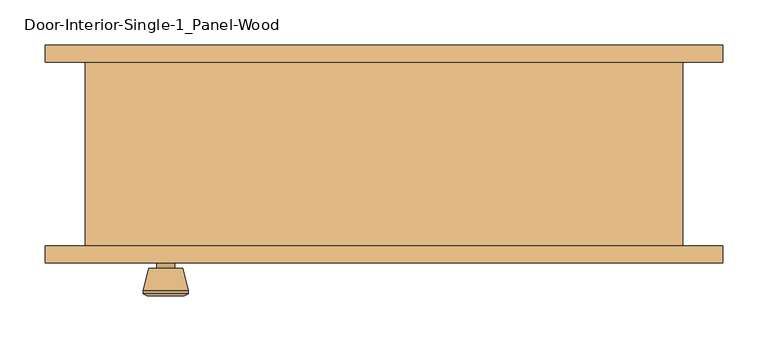
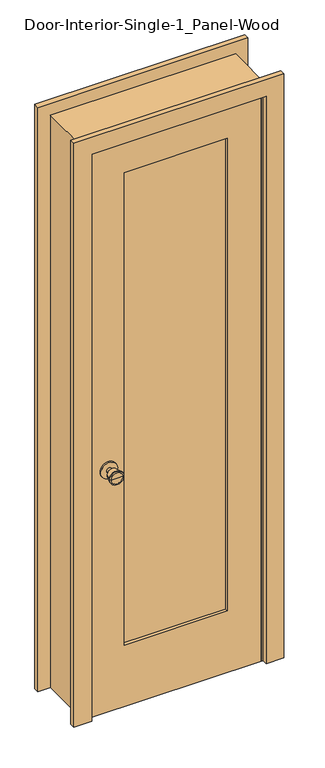
"""IFC4 building model written with IfcOpenShell, lengths in millimetres: door geometry, Door-Interior-Single-1_Panel-Wood."""

from ifc_helpers import new_model, si_unit, point, frame, frame_2d, origin, place, context, project, spatial, polyline, circle_curve, trimmed, segment, composite_curve, outline, extrude, faceted_brep, source, transform, mapped, element, save
from ifc_brep_helpers import plane_surface, cylinder_surface, revolved_surface, advanced_brep


def door_interior_single_1_panel_wood_a1a047a4(model_context):
    return source(origin(), model_context, "Body", "SolidModel", [
        advanced_brep(
        [(-241.3, -57.5, 914.4), (-251.3, -57.5, 914.4), (-231.3, -57.5, 914.4), (-220.8241324, -8.5, 914.4), (-261.7758676, -8.5, 914.4), (-241.3, -8.5, 914.4), (-216.3, -10.3278681, 914.4), (-266.3, -10.3278681, 914.4), (-216.3, -13.7915463, 914.4), (-266.3, -13.7915463, 914.4), (-222.663764, -38.5, 914.4), (-259.936236, -38.5, 914.4), (-231.3, -38.5, 914.4), (-251.3, -38.5, 914.4)],
        [
            (0, 1),
            (1, 2, circle_curve(frame((-241.3, -57.5, 914.4), z_axis=(0.0, -1.0, 0.0), x_axis=(-1.0, 0.0, 0.0)), 10.0)),
            (2, 0),
            (2, 1, circle_curve(frame((-241.3, -57.5, 914.4), z_axis=(0.0, -1.0, 0.0), x_axis=(-1.0, 0.0, 0.0)), 10.0)),
            (3, 4, circle_curve(frame((-241.3, -8.5, 914.4), z_axis=(0.0, 1.0, 0.0), x_axis=(-1.0, 0.0, 0.0)), 20.4758676)),
            (4, 5),
            (5, 3),
            (4, 3, circle_curve(frame((-241.3, -8.5, 914.4), z_axis=(0.0, 1.0, 0.0), x_axis=(-1.0, 0.0, 0.0)), 20.4758676)),
            (6, 7, circle_curve(frame((-241.3, -10.3278681, 914.4), z_axis=(0.0, 1.0, 0.0), x_axis=(-1.0, 0.0, 0.0)), 25.0)),
            (7, 4),
            (3, 6),
            (7, 6, circle_curve(frame((-241.3, -10.3278681, 914.4), z_axis=(0.0, 1.0, 0.0), x_axis=(-1.0, 0.0, 0.0)), 25.0)),
            (8, 9, circle_curve(frame((-241.3, -13.7915463, 914.4), z_axis=(0.0, 1.0, 0.0), x_axis=(-1.0, 0.0, 0.0)), 25.0)),
            (9, 7),
            (6, 8),
            (9, 8, circle_curve(frame((-241.3, -13.7915463, 914.4), z_axis=(0.0, 1.0, 0.0), x_axis=(-1.0, 0.0, 0.0)), 25.0)),
            (10, 11, circle_curve(frame((-241.3, -38.5, 914.4), z_axis=(0.0, 1.0, 0.0), x_axis=(-1.0, 0.0, 0.0)), 18.636236)),
            (11, 9),
            (8, 10),
            (11, 10, circle_curve(frame((-241.3, -38.5, 914.4), z_axis=(0.0, 1.0, 0.0), x_axis=(-1.0, 0.0, 0.0)), 18.636236)),
            (12, 13, circle_curve(frame((-241.3, -38.5, 914.4), z_axis=(0.0, 1.0, 0.0), x_axis=(-1.0, 0.0, 0.0)), 10.0)),
            (13, 11),
            (10, 12),
            (13, 12, circle_curve(frame((-241.3, -38.5, 914.4), z_axis=(0.0, 1.0, 0.0), x_axis=(-1.0, 0.0, 0.0)), 10.0)),
            (1, 13),
            (12, 2),
        ],
        [
            plane_surface(frame((-241.3, -57.5, 914.4), z_axis=(0.0, -1.0, 0.0), x_axis=(-1.0, 0.0, 0.0))),
            plane_surface(frame((-241.3, -8.5, 914.4), z_axis=(0.0, 1.0, 0.0), x_axis=(-1.0, 0.0, 0.0))),
            revolved_surface(polyline([(-261.7758676, -8.5, 914.4), (-266.3, -10.3278681, 914.4)]), (-241.3, -57.5, 914.4), (0.0, -1.0, 0.0)),
            cylinder_surface(frame((-241.3, -57.5, 914.4), z_axis=(0.0, -1.0, 0.0), x_axis=(-1.0, 0.0, 0.0)), 25.0),
            revolved_surface(polyline([(-266.3, -13.7915463, 914.4), (-259.936236, -38.5, 914.4)]), (-241.3, -57.5, 914.4), (0.0, -1.0, 0.0)),
            plane_surface(frame((-241.3, -38.5, 914.4), z_axis=(0.0, -1.0, 0.0), x_axis=(-1.0, 0.0, 0.0))),
            cylinder_surface(frame((-241.3, -57.5, 914.4), z_axis=(0.0, -1.0, 0.0), x_axis=(-1.0, 0.0, 0.0)), 10.0),
        ],
        [
            (0, [[1, 2, 3]]),
            (0, [[-3, 4, -1]]),
            (1, [[5, 6, 7]]),
            (1, [[8, -7, -6]]),
            (2, [[9, 10, -5, 11]]),
            (2, [[12, -11, -8, -10]]),
            (3, [[13, 14, -9, 15]]),
            (3, [[16, -15, -12, -14]]),
            (4, [[17, 18, -13, 19]]),
            (4, [[20, -19, -16, -18]]),
            (5, [[21, 22, -17, 23]]),
            (5, [[24, -23, -20, -22]]),
            (6, [[-2, 25, -21, 26]]),
            (6, [[-4, -26, -24, -25]]),
        ],
    ),
        extrude(outline(composite_curve([segment(trimmed(circle_curve(frame_2d((914.4, -241.3)), 30.0), [point((914.4, -271.3))], [point((914.4, -211.3))], False, "CARTESIAN"), True, "CONTINUOUS"), segment(trimmed(circle_curve(frame_2d((914.4, -241.3)), 30.0), [point((914.4, -211.3))], [point((914.4, -271.3))], False, "CARTESIAN"), True, "CONTINUOUS")], self_intersect=False)), frame((0.0, -63.5, 0.0), z_axis=(0.0, 1.0, 0.0), x_axis=(0.0, 0.0, 1.0)), (0.0, 0.0, 1.0), 6.0),
        advanced_brep(
        [(-241.3, -104.425, 914.4), (-231.3, -104.425, 914.4), (-251.3, -104.425, 914.4), (-220.8241324, -153.425, 914.4), (-241.3, -153.425, 914.4), (-261.7758676, -153.425, 914.4), (-216.3, -151.5971319, 914.4), (-266.3, -151.5971319, 914.4), (-216.3, -148.1334537, 914.4), (-266.3, -148.1334537, 914.4), (-222.663764, -123.425, 914.4), (-259.936236, -123.425, 914.4), (-231.3, -123.425, 914.4), (-251.3, -123.425, 914.4)],
        [
            (0, 1),
            (1, 2, circle_curve(frame((-241.3, -104.425, 914.4), z_axis=(0.0, 1.0, 0.0), x_axis=(-1.0, 0.0, 0.0)), 10.0)),
            (2, 0),
            (2, 1, circle_curve(frame((-241.3, -104.425, 914.4), z_axis=(0.0, 1.0, 0.0), x_axis=(-1.0, 0.0, 0.0)), 10.0)),
            (3, 4),
            (4, 5),
            (5, 3, circle_curve(frame((-241.3, -153.425, 914.4), z_axis=(0.0, -1.0, 0.0), x_axis=(-1.0, 0.0, 0.0)), 20.4758676)),
            (3, 5, circle_curve(frame((-241.3, -153.425, 914.4), z_axis=(0.0, -1.0, 0.0), x_axis=(-1.0, 0.0, 0.0)), 20.4758676)),
            (6, 3),
            (5, 7),
            (7, 6, circle_curve(frame((-241.3, -151.5971319, 914.4), z_axis=(0.0, -1.0, 0.0), x_axis=(-1.0, 0.0, 0.0)), 25.0)),
            (6, 7, circle_curve(frame((-241.3, -151.5971319, 914.4), z_axis=(0.0, -1.0, 0.0), x_axis=(-1.0, 0.0, 0.0)), 25.0)),
            (8, 6),
            (7, 9),
            (9, 8, circle_curve(frame((-241.3, -148.1334537, 914.4), z_axis=(0.0, -1.0, 0.0), x_axis=(-1.0, 0.0, 0.0)), 25.0)),
            (8, 9, circle_curve(frame((-241.3, -148.1334537, 914.4), z_axis=(0.0, -1.0, 0.0), x_axis=(-1.0, 0.0, 0.0)), 25.0)),
            (10, 8),
            (9, 11),
            (11, 10, circle_curve(frame((-241.3, -123.425, 914.4), z_axis=(0.0, -1.0, 0.0), x_axis=(-1.0, 0.0, 0.0)), 18.636236)),
            (10, 11, circle_curve(frame((-241.3, -123.425, 914.4), z_axis=(0.0, -1.0, 0.0), x_axis=(-1.0, 0.0, 0.0)), 18.636236)),
            (12, 10),
            (11, 13),
            (13, 12, circle_curve(frame((-241.3, -123.425, 914.4), z_axis=(0.0, -1.0, 0.0), x_axis=(-1.0, 0.0, 0.0)), 10.0)),
            (12, 13, circle_curve(frame((-241.3, -123.425, 914.4), z_axis=(0.0, -1.0, 0.0), x_axis=(-1.0, 0.0, 0.0)), 10.0)),
            (1, 12),
            (13, 2),
        ],
        [
            plane_surface(frame((-241.3, -104.425, 914.4), z_axis=(0.0, 1.0, 0.0), x_axis=(-1.0, 0.0, 0.0))),
            plane_surface(frame((-241.3, -153.425, 914.4), z_axis=(0.0, -1.0, 0.0), x_axis=(-1.0, 0.0, 0.0))),
            revolved_surface(polyline([(-261.7758676, -153.425, 914.4), (-266.3, -151.5971319, 914.4)]), (-241.3, -104.425, 914.4), (0.0, 1.0, 0.0)),
            cylinder_surface(frame((-241.3, -104.425, 914.4), z_axis=(0.0, 1.0, 0.0), x_axis=(-1.0, 0.0, 0.0)), 25.0),
            revolved_surface(polyline([(-266.3, -148.1334537, 914.4), (-259.936236, -123.425, 914.4)]), (-241.3, -104.425, 914.4), (0.0, 1.0, 0.0)),
            plane_surface(frame((-241.3, -123.425, 914.4), z_axis=(0.0, 1.0, 0.0), x_axis=(-1.0, 0.0, 0.0))),
            cylinder_surface(frame((-241.3, -104.425, 914.4), z_axis=(0.0, 1.0, 0.0), x_axis=(-1.0, 0.0, 0.0)), 10.0),
        ],
        [
            (0, [[1, 2, 3]]),
            (0, [[-3, 4, -1]]),
            (1, [[5, 6, 7]]),
            (1, [[-6, -5, 8]]),
            (2, [[9, -7, 10, 11]]),
            (2, [[-10, -8, -9, 12]]),
            (3, [[13, -11, 14, 15]]),
            (3, [[-14, -12, -13, 16]]),
            (4, [[17, -15, 18, 19]]),
            (4, [[-18, -16, -17, 20]]),
            (5, [[21, -19, 22, 23]]),
            (5, [[-22, -20, -21, 24]]),
            (6, [[25, -23, 26, -2]]),
            (6, [[-26, -24, -25, -4]]),
        ],
    ),
        extrude(outline(composite_curve([segment(trimmed(circle_curve(frame_2d((914.4, -241.3)), 30.0), [point((914.4, -271.3))], [point((914.4, -211.3))], False, "CARTESIAN"), True, "CONTINUOUS"), segment(trimmed(circle_curve(frame_2d((914.4, -241.3)), 30.0), [point((914.4, -211.3))], [point((914.4, -271.3))], False, "CARTESIAN"), True, "CONTINUOUS")], self_intersect=False)), frame((0.0, -104.425, 0.0), z_axis=(0.0, 1.0, 0.0), x_axis=(0.0, 0.0, 1.0)), (0.0, 0.0, 1.0), 6.0),
        faceted_brep([(330.2, -98.425, 0.0), (304.8, -98.425, 0.0), (304.8, -63.5, 0.0), (292.1, -63.5, 0.0), (292.1, -28.575, 0.0), (304.8, -28.575, 0.0), (304.8, 104.775, 0.0), (330.2, 104.775, 0.0), (330.2, 104.775, 2159.0), (330.2, -98.425, 2159.0), (304.8, 104.775, 2133.6), (-304.8, 104.775, 2133.6), (-304.8, 104.775, 0.0), (-330.2, 104.775, 0.0), (-330.2, 104.775, 2159.0), (304.8, -28.575, 2133.6), (292.1, -28.575, 2120.9), (-292.1, -28.575, 2120.9), (-292.1, -28.575, 0.0), (-304.8, -28.575, 0.0), (-304.8, -28.575, 2133.6), (292.1, -63.5, 2120.9), (304.8, -63.5, 2133.6), (-304.8, -63.5, 2133.6), (-304.8, -63.5, 0.0), (-292.1, -63.5, 0.0), (-292.1, -63.5, 2120.9), (304.8, -98.425, 2133.6), (-330.2, -98.425, 2159.0), (-330.2, -98.425, 0.0), (-304.8, -98.425, 0.0), (-304.8, -98.425, 2133.6)], [[[0, 1, 2, 3, 4, 5, 6, 7]], [[7, 8, 9, 0]], [[6, 10, 11, 12, 13, 14, 8, 7]], [[5, 15, 10, 6]], [[4, 16, 17, 18, 19, 20, 15, 5]], [[3, 21, 16, 4]], [[2, 22, 23, 24, 25, 26, 21, 3]], [[1, 27, 22, 2]], [[0, 9, 28, 29, 30, 31, 27, 1]], [[8, 14, 28, 9]], [[15, 20, 11, 10]], [[21, 26, 17, 16]], [[27, 31, 23, 22]], [[29, 13, 12, 19, 18, 25, 24, 30]], [[14, 13, 29, 28]], [[20, 19, 12, 11]], [[26, 25, 18, 17]], [[31, 30, 24, 23]]]),
        extrude(outline(polyline([(2133.6, -304.8), (0.0, -304.8), (0.0, 304.8), (2133.6, 304.8), (2133.6, -304.8)]), holes=[polyline([(2014.5375, -184.15), (2014.5375, 184.15), (231.775, 184.15), (231.775, -184.15), (2014.5375, -184.15)])]), frame((0.0, -98.425, 0.0), z_axis=(0.0, 1.0, 0.0), x_axis=(0.0, 0.0, 1.0)), (0.0, 0.0, 1.0), 34.925),
        extrude(outline(polyline([(184.15, -75.1416667), (184.15, -86.7833333), (-184.15, -86.7833333), (-184.15, -75.1416667), (184.15, -75.1416667)])), frame((0.0, 0.0, 231.775), z_axis=(0.0, 0.0, 1.0), x_axis=(1.0, 0.0, 0.0)), (0.0, 0.0, 1.0), 1782.7625),
        extrude(outline(polyline([(0.0, 374.65), (2203.45, 374.65), (2203.45, -374.65), (0.0, -374.65), (0.0, -311.15), (2139.95, -311.15), (2139.95, 311.15), (0.0, 311.15), (0.0, 374.65)])), frame((0.0, -117.475, 0.0), z_axis=(0.0, 1.0, 0.0), x_axis=(0.0, 0.0, 1.0)), (0.0, 0.0, 1.0), 19.05),
        extrude(outline(polyline([(0.0, 374.65), (2203.45, 374.65), (2203.45, -374.65), (0.0, -374.65), (0.0, -311.15), (2139.95, -311.15), (2139.95, 311.15), (0.0, 311.15), (0.0, 374.65)])), frame((0.0, 104.775, 0.0), z_axis=(0.0, 1.0, 0.0), x_axis=(0.0, 0.0, 1.0)), (0.0, 0.0, 1.0), 19.05),
    ])


if __name__ == "__main__":
    model = new_model("IFC4")
    model_context = context("Model", 3, world=origin())
    ifc_project = project(units=[si_unit("LENGTHUNIT", "METRE", prefix="MILLI")], contexts=[model_context])
    site = spatial("IfcSite", under=ifc_project)
    building = spatial("IfcBuilding", under=site)
    placement = place(None, origin())
    door_interior_single_1_panel_wood_shape = door_interior_single_1_panel_wood_a1a047a4(model_context)
    element("IfcDoor", 1, ObjectType="Door-Interior-Single-1_Panel-Wood", at=placement, inside=building, context=model_context, shape_type="MappedRepresentation", body=[
        mapped(door_interior_single_1_panel_wood_shape, transform((0.0, 0.0, 0.0), x_axis=(1.0, 0.0, 0.0), y_axis=(0.0, 1.0, 0.0), z_axis=(0.0, 0.0, 1.0))),
    ])
    save(model, "model.ifc")

# Revit data of these elements
# Type "Door-Interior-Single-1_Panel-Wood"
#   Type Mark = "12"
#   Assembly Code = "C1020300"
#   Analytic Construction = "Wooden"
#   Top Rail = 0' - 4 11/16"
#   Thickness = 0' - 1 3/8"
#   Thermal Resistance (R) = 2.5876 (h·ft²·°F)/BTU
#   Swing Angle [instance default] = 90.00°
#   Stiles = 0' - 4 3/4"
#   Rough Width = 2' - 2"
#   Rough Height = 7' - 1"
#   Height = 7' - 0"
#   Width = 2' - 0"
#   Heat Transfer Coefficient (U) = 0.3865 BTU/(h·ft²·°F)
#   Bottom Rail = 0' - 9 1/8"
#   Trim Material = Cherry
#   Panel Material = Cherry
#   Frame Material = Cherry
#   Door Handle Material = Aluminum
#   Visual Light Transmittance = 0
#   Solar Heat Gain Coefficient = 0
#   Wall Closure = (empty or 0)
#   Function = (empty or 0)
# Element 1 (IfcDoor, "Door-Interior-Single-1_Panel-Wood")
#   Materials on its faces: "Cherry", "Aluminum"
# Materials
#   "Cherry": class "Wood", colour RGB 226 177 128, transparency 0, Description = "Prunus Serotina", Cost = 0
#   "Aluminum": class "Metal", colour RGB 247 247 247, transparency 0, Description = "Aluminum 6061", Cost = 0
